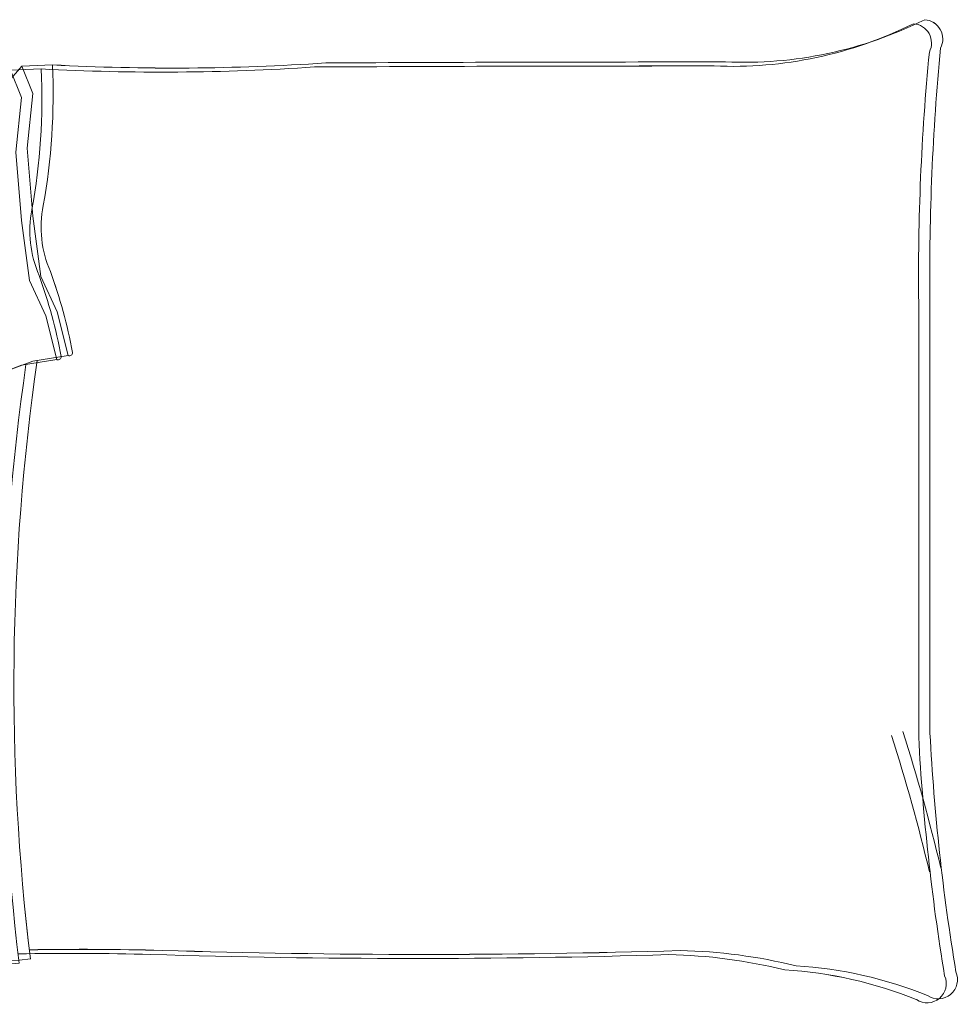
# Model space of a CAD drawing. Units: inches. Extents: x 1962 to 2771, y 1245 to 2660.
# Tile 27 of 114: x 2116 to 2158, y 1849 to 1893. Entities that reach past the tile are written whole.
import ezdxf

# ---------------------------------------------------------------- set-up
doc = ezdxf.new("R2010")
doc.units = ezdxf.units.IN
doc.layers.add('A-FURN', color=8, linetype='Continuous', lineweight=13)

# ---------------------------------------------------------------- blocks, each defined once
blk = doc.blocks.new('BED-PLAN')
for p, q in [((22.563, 42.207), (19.979, 39.261)), ((22.563, 42.206), (19.979, 39.261)), ((23.95, 42.27), (22.563, 42.207, 3.077)), ((23.95, 42.27), (22.563, 42.206, 3.077)), ((23.055, 40.985), (22.563, 42.207)), ((23.055, 40.985), (22.563, 42.206)), ((22.055, 42.025), (19.471, 39.08)), ((22.055, 42.025), (19.471, 39.08)), ((23.442, 42.088), (22.055, 42.025, 3.077)), ((23.442, 42.088), (22.055, 42.025, 3.077)), ((22.547, 40.803), (22.055, 42.025)), ((22.547, 40.803), (22.055, 42.025)), ((0.508, 40.933), (21.66, 40.933)), ((0.508, 40.933), (21.66, 40.933)), ((1.727, 2.945), (1.727, 40.933)), ((1.727, 2.945), (1.727, 40.933)), ((22.809, 38.523), (23.055, 40.985)), ((22.809, 38.522), (23.055, 40.985)), ((0, 40.752), (21.152, 40.752)), ((0, 40.751), (21.152, 40.751)), ((0, 2.764), (0, 40.751)), ((1.219, 2.764), (1.219, 40.752)), ((1.219, 2.763), (1.219, 40.751)), ((13.682, 40.482), (11.187, 39.866)), ((13.682, 40.482), (11.187, 39.866)), ((13.361, 36.403), (13.682, 40.482)), ((13.361, 36.403), (13.682, 40.482)), ((22.301, 38.341), (22.547, 40.803)), ((22.301, 38.341), (22.547, 40.803)), ((2.541, 40.016), (2.464, 35.722)), ((2.541, 40.016), (2.464, 35.722)), ((2.541, 40.016), (5.093, 39.715)), ((2.541, 40.016), (5.093, 39.715)), ((4.585, 39.534), (6.628, 40.007)), ((4.585, 39.533), (6.628, 40.007)), ((5.093, 39.715), (7.136, 40.188)), ((5.093, 39.715), (7.136, 40.188)), ((6.628, 40.007), (7.46, 39.598)), ((6.628, 40.007), (7.46, 39.598)), ((9.911, 40.016), (7.072, 39.378)), ((9.911, 40.016), (7.072, 39.378)), ((7.136, 40.188), (7.968, 39.78)), ((7.136, 40.188), (7.968, 39.78)), ((11.187, 39.866), (9.911, 40.016)), ((11.187, 39.866), (9.911, 40.016)), ((13.173, 40.301), (10.679, 39.684)), ((13.173, 40.301), (10.679, 39.684)), ((12.853, 36.222), (13.173, 40.301)), ((12.853, 36.221), (13.173, 40.301)), ((2.033, 39.835), (1.955, 35.54)), ((2.033, 39.834), (1.956, 35.54)), ((2.033, 39.835), (4.585, 39.534)), ((2.033, 39.834), (4.585, 39.533)), ((9.402, 39.835), (6.563, 39.197)), ((9.402, 39.835), (6.563, 39.197)), ((10.679, 39.684), (9.402, 39.835)), ((10.679, 39.684), (9.402, 39.835)), ((6.563, 39.197), (4.434, 38.258)), ((6.563, 39.197), (4.434, 38.258)), ((7.072, 39.378), (4.942, 38.439)), ((7.072, 39.378), (4.942, 38.439)), ((19.471, 39.08), (17.749, 36.741)), ((19.471, 39.08), (17.749, 36.741)), ((19.979, 39.261), (18.257, 36.922)), ((19.979, 39.261), (18.257, 36.922)), ((22.547, 35.263), (22.301, 38.341)), ((22.547, 35.263), (22.301, 38.341)), ((23.055, 35.445), (22.809, 38.523)), ((23.055, 35.445), (22.809, 38.522)), ((18.257, 36.922), (16.658, 32.49)), ((18.257, 36.922), (16.658, 32.49)), ((2.464, 35.722), (2.529, 36.519)), ((2.464, 35.722), (2.529, 36.519)), ((2.529, 36.519), (2.948, 33.5)), ((2.529, 36.519), (2.948, 33.5)), ((13.804, 34.845), (13.361, 36.403)), ((13.804, 34.845), (13.361, 36.403)), ((17.749, 36.741), (16.149, 32.309)), ((17.749, 36.741), (16.149, 32.309)), ((1.955, 35.54), (2.021, 36.338)), ((1.956, 35.54), (2.021, 36.337)), ((2.021, 36.338), (2.44, 33.319)), ((2.021, 36.337), (2.44, 33.318)), ((13.296, 34.663), (12.853, 36.222)), ((13.296, 34.663), (12.853, 36.221)), ((22.916, 32.555), (22.547, 35.263)), ((22.916, 32.555), (22.547, 35.263)), ((23.424, 32.737), (23.055, 35.445)), ((23.424, 32.736), (23.055, 35.445)), ((12.953, 29.091), (13.296, 34.663)), ((12.953, 29.091), (13.296, 34.663)), ((13.461, 29.273), (13.804, 34.845)), ((13.461, 29.273), (13.804, 34.845)), ((2.44, 33.319), (3.515, 29.011)), ((2.44, 33.318), (3.515, 29.011)), ((2.948, 33.5), (4.023, 29.192)), ((2.948, 33.5), (4.023, 29.192)), ((16.658, 32.49), (14.326, 25.863)), ((16.658, 32.49), (14.326, 25.862)), ((23.654, 30.955), (22.916, 32.555)), ((23.654, 30.955), (22.916, 32.555)), ((24.162, 31.136), (23.424, 32.737)), ((24.162, 31.136), (23.424, 32.736)), ((16.149, 32.309), (13.818, 25.681)), ((16.149, 32.309), (13.818, 25.681)), ((62.991, 11.975), (62.991, 31.54)), ((62.991, 11.975), (62.991, 31.54)), ((63.499, 12.157), (63.499, 31.722)), ((63.499, 12.156), (63.499, 31.722)), ((2.92, 31.161), (2.447, 29.52)), ((2.92, 31.161), (2.447, 29.519)), ((3.428, 31.343), (2.955, 29.701)), ((3.428, 31.342), (2.955, 29.701)), ((24.655, 29.167), (24.162, 31.136)), ((24.655, 29.166), (24.162, 31.136)), ((24.146, 28.985), (23.654, 30.955)), ((24.146, 28.985), (23.654, 30.955)), ((2.447, 29.52), (2.017, 27.19)), ((2.447, 29.519), (2.017, 27.19)), ((2.955, 29.701), (2.525, 27.372)), ((2.955, 29.701), (2.525, 27.372)), ((12.423, 25.886), (12.953, 29.091)), ((12.423, 25.886), (12.953, 29.091)), ((12.931, 26.068), (13.461, 29.273)), ((12.931, 26.068), (13.461, 29.273)), ((19.487, 27.566), (23.055, 28.92)), ((19.487, 27.566), (23.055, 28.92)), ((22.547, 28.739), (24.146, 28.985)), ((22.547, 28.739), (24.146, 28.985)), ((23.055, 28.92), (24.655, 29.167)), ((23.055, 28.92), (24.655, 29.166)), ((18.979, 27.385), (22.547, 28.739)), ((18.979, 27.384), (22.547, 28.739)), ((14.326, 24.236), (19.487, 27.566)), ((14.326, 24.235), (19.487, 27.566)), ((2.017, 27.19), (2.033, 26.935)), ((2.017, 27.19), (2.033, 26.935)), ((2.525, 27.372), (2.541, 27.117)), ((2.525, 27.372), (2.541, 27.116)), ((2.541, 27.117), (2.876, 23.597)), ((2.541, 27.116), (2.876, 23.597)), ((13.818, 24.054), (18.979, 27.385)), ((13.818, 24.054), (18.979, 27.384)), ((2.033, 26.935), (2.368, 23.415)), ((2.033, 26.935), (2.368, 23.415)), ((13.306, 24.444), (12.285, 26.885)), ((13.306, 24.444), (12.285, 26.885)), ((13.814, 24.626), (12.793, 27.067)), ((13.814, 24.626), (12.793, 27.066)), ((13.428, 22.495), (13.306, 24.444)), ((13.428, 22.495), (13.306, 24.444)), ((13.936, 22.676), (13.814, 24.626)), ((13.936, 22.676), (13.814, 24.626)), ((2.876, 23.597), (2.489, 22.421)), ((2.876, 23.597), (2.489, 22.421)), ((2.368, 23.415), (1.981, 22.24)), ((2.368, 23.415), (1.981, 22.24)), ((11.809, 22.543), (13.936, 22.676)), ((11.809, 22.543), (13.936, 22.676)), ((1.981, 22.24), (6.254, 22.046)), ((1.981, 22.24), (6.254, 22.046)), ((2.489, 22.421), (6.762, 22.228)), ((2.489, 22.421), (6.762, 22.228)), ((6.762, 22.228), (9.314, 21.927)), ((6.762, 22.228), (9.314, 21.927)), ((9.838, 21.81), (11.301, 22.362)), ((9.838, 21.81), (11.301, 22.362)), ((10.346, 21.991), (11.809, 22.543)), ((10.346, 21.991), (11.809, 22.543)), ((11.301, 22.362), (13.428, 22.495)), ((11.301, 22.362), (13.428, 22.495)), ((6.247, 21.296), (8.776, 21.755)), ((6.247, 21.296), (8.776, 21.755)), ((6.254, 22.046), (8.806, 21.745)), ((6.254, 22.046), (8.806, 21.745)), ((8.776, 21.755), (9.81, 21.755)), ((8.776, 21.755), (9.81, 21.755)), ((8.806, 21.745), (9.838, 21.81)), ((8.806, 21.745), (9.838, 21.81)), ((9.314, 21.927), (10.346, 21.991)), ((9.314, 21.927), (10.346, 21.991)), ((9.81, 21.755), (11.304, 21.296)), ((9.81, 21.755), (11.304, 21.296)), ((5.739, 21.114), (8.268, 21.574)), ((5.739, 21.114), (8.268, 21.574)), ((8.268, 21.574), (9.302, 21.574)), ((8.268, 21.574), (9.302, 21.574)), ((9.302, 21.574), (10.796, 21.114)), ((9.302, 21.574), (10.796, 21.114)), ((1.487, 20.655), (5.739, 21.114)), ((1.487, 20.654), (5.739, 21.114)), ((1.995, 20.836), (6.247, 21.296)), ((1.995, 20.836), (6.247, 21.296)), ((10.796, 21.114), (12.927, 21.114)), ((10.796, 21.114), (12.927, 21.114)), ((11.304, 21.296), (13.436, 21.296)), ((11.304, 21.296), (13.436, 21.296)), ((12.927, 21.114), (12.927, 19.161)), ((12.927, 21.114), (12.927, 19.161)), ((13.436, 21.296), (13.436, 19.342)), ((13.436, 21.296), (13.436, 19.342)), ((1.946, 19.506), (1.487, 20.655)), ((1.946, 19.505), (1.487, 20.654)), ((2.455, 19.687), (1.995, 20.836)), ((2.455, 19.687), (1.995, 20.836)), ((2.34, 16.153), (2.455, 19.687)), ((2.34, 16.153), (2.455, 19.687)), ((13.361, 15.591), (13.682, 19.67)), ((13.361, 15.591), (13.682, 19.67)), ((1.831, 15.972), (1.946, 19.506)), ((1.831, 15.972), (1.946, 19.505)), ((12.927, 19.161), (12.06, 16.661)), ((12.927, 19.161), (12.06, 16.661)), ((13.436, 19.342), (12.568, 16.843)), ((13.436, 19.342), (12.568, 16.843)), ((12.853, 15.409), (13.173, 19.489)), ((12.853, 15.409), (13.173, 19.488)), ((2.34, 15.898), (2.34, 16.153)), ((2.34, 15.897), (2.34, 16.153)), ((1.831, 15.716), (1.831, 15.972)), ((1.831, 15.716), (1.831, 15.972)), ((2.406, 13.418), (1.831, 15.716)), ((2.406, 13.418), (1.831, 15.716)), ((2.914, 13.6), (2.34, 15.898)), ((2.914, 13.599), (2.34, 15.897)), ((13.804, 14.033), (13.361, 15.591)), ((13.804, 14.032), (13.361, 15.591)), ((13.296, 13.851), (12.853, 15.409)), ((13.296, 13.851), (12.853, 15.409)), ((2.636, 9.626), (3.44, 13.993)), ((2.636, 9.626), (3.44, 13.992)), ((3.144, 9.808), (3.949, 14.174)), ((3.144, 9.807), (3.949, 14.174)), ((12.953, 8.279), (13.296, 13.851)), ((12.953, 8.279), (13.296, 13.851)), ((13.461, 8.461), (13.804, 14.033)), ((13.461, 8.46), (13.804, 14.032)), ((2.981, 11.809), (2.406, 13.418)), ((2.981, 11.809), (2.406, 13.418)), ((3.489, 11.991), (2.914, 13.6)), ((3.489, 11.991), (2.914, 13.599)), ((2.914, 6.768), (3.144, 9.808)), ((2.914, 6.768), (3.144, 9.807)), ((2.406, 6.587), (2.636, 9.626)), ((2.406, 6.587), (2.636, 9.626)), ((12.931, 5.256), (13.461, 8.461)), ((12.931, 5.255), (13.461, 8.46)), ((13.461, 8.461), (13.718, 7.56)), ((13.461, 8.46), (13.718, 7.56)), ((12.423, 5.074), (12.953, 8.279)), ((12.423, 5.074), (12.953, 8.279)), ((12.953, 8.279), (13.21, 7.378)), ((12.953, 8.279), (13.21, 7.378)), ((13.718, 7.56), (14.292, 3.509)), ((13.718, 7.56), (14.292, 3.508)), ((13.21, 7.378), (13.784, 3.327)), ((13.21, 7.378), (13.784, 3.327)), ((2.9, 6.685), (2.914, 6.768)), ((2.9, 6.684), (2.914, 6.768)), ((3.162, 3.282), (2.9, 6.685)), ((3.162, 3.282), (2.9, 6.684)), ((2.392, 6.503), (2.406, 6.587)), ((2.392, 6.503), (2.406, 6.587)), ((2.653, 3.1), (2.392, 6.503)), ((2.653, 3.1), (2.392, 6.503)), ((7.626, 4.198), (5.443, 5.002)), ((7.626, 4.198), (5.443, 5.002)), ((7.118, 4.016), (4.935, 4.821)), ((7.118, 4.016), (4.935, 4.821)), ((9.991, 3.557), (7.118, 4.016)), ((9.992, 3.557), (7.118, 4.016)), ((10.5, 3.738), (7.626, 4.198)), ((10.5, 3.738), (7.626, 4.198)), ((2.636, 3.097), (5.164, 3.557)), ((2.636, 3.097), (5.164, 3.557)), ((3.144, 3.279), (5.673, 3.738)), ((3.144, 3.279), (5.673, 3.738)), ((5.164, 3.557), (7.233, 3.212)), ((5.164, 3.557), (7.233, 3.212)), ((5.673, 3.738), (7.741, 3.394)), ((5.673, 3.738), (7.741, 3.393)), ((7.233, 3.212), (8.038, 3.672)), ((7.233, 3.212), (8.038, 3.672)), ((7.741, 3.394), (8.546, 3.853)), ((7.741, 3.393), (8.546, 3.853)), ((11.256, 3.787), (9.991, 3.557)), ((11.256, 3.786), (9.992, 3.557)), ((11.764, 3.968), (10.5, 3.738)), ((11.764, 3.968), (10.5, 3.738)), ((13.784, 3.327), (11.256, 3.787)), ((13.784, 3.327), (11.256, 3.786)), ((14.292, 3.509), (11.764, 3.968)), ((14.292, 3.508), (11.764, 3.968)), ((14.396, 2.764), (0, 2.764)), ((14.396, 2.763), (0, 2.763)), ((14.904, 2.945), (0.508, 2.945)), ((14.904, 2.945), (0.508, 2.945))]:
    blk.add_line(p, q)
for centre, radius, start, end in [((54.582, 60.538), 18.334, 267.4714, 296.4681), ((54.582, 60.538), 18.334, 267.4714, 296.4681), ((55.09, 60.719), 18.334, 267.4714, 296.4681), ((55.09, 60.719), 18.334, 267.4714, 296.4681), ((62.693, 43.251), 0.876, 332.6588, 86.02), ((62.693, 43.251), 0.876, 332.6588, 86.02), ((63.201, 43.433), 0.876, 332.6588, 86.02), ((63.201, 43.432), 0.876, 332.6588, 86.02), ((168.736, 32.712), 105.752, 174.4998, 180.63509), ((168.736, 32.712), 105.752, 174.4998, 180.63509), ((169.244, 32.894), 105.752, 174.4998, 180.63509), ((169.244, 32.894), 105.752, 174.4998, 180.63509), ((28.866, 144.882), 102.937, 266.97912, 273.83645), ((28.866, 144.882), 102.937, 266.97912, 273.83645), ((-4.783, 40.982), 28.761, 349.8763, 2.5657), ((-4.783, 40.982), 28.761, 349.8763, 2.5657), ((29.375, 145.064), 102.937, 266.97912, 273.83645), ((29.375, 145.063), 102.937, 266.97912, 273.83645), ((53.91, -3583.936), 3626.158, 90.002168, 90.286887), ((53.91, -3583.937), 3626.158, 90.002168, 90.286887), ((54.419, -3583.755), 3626.158, 90.002168, 90.286887), ((54.419, -3583.755), 3626.158, 90.002168, 90.286887), ((-5.291, 40.801), 28.761, 349.8763, 2.5657), ((-5.291, 40.801), 28.761, 349.8763, 2.5657), ((27.874, 34.772), 4.948, 168.6608, 203.7384), ((27.874, 34.772), 4.948, 168.6608, 203.7384), ((28.382, 34.954), 4.948, 168.6608, 203.7384), ((28.382, 34.954), 4.948, 168.6608, 203.7384), ((1.686, 24.947), 23.571, 10.6617, 19.8806), ((1.686, 24.946), 23.571, 10.6617, 19.8806), ((1.178, 24.765), 23.571, 10.6617, 19.8806), ((1.178, 24.765), 23.571, 10.6617, 19.8806), ((24.704, 29.305), 0.147, 250.2464, 1.1377), ((24.704, 29.304), 0.147, 250.2464, 1.1377), ((124.762, 14.297), 102.556, 171.78449, 186.90062), ((124.762, 14.296), 102.556, 171.78449, 186.90062), ((24.196, 29.123), 0.147, 250.2464, 1.1377), ((24.196, 29.123), 0.147, 250.2464, 1.1377), ((124.254, 14.115), 102.556, 171.78449, 186.90062), ((124.254, 14.115), 102.556, 171.78449, 186.90062), ((144.711, 16.979), 131.131, 176.08655, 186.78213), ((144.711, 16.979), 131.131, 176.08655, 186.78213), ((145.219, 17.161), 131.131, 176.08655, 186.78213), ((145.219, 17.161), 131.131, 176.08655, 186.78213), ((-18.848, -13.688), 84.623, 13.38322, 17.70533), ((-18.848, -13.688), 84.623, 13.38322, 17.70533), ((-18.34, -13.506), 84.623, 13.38322, 17.70533), ((-18.34, -13.507), 84.623, 13.38322, 17.70533), ((160.151, 17.215), 96.784, 182.99578, 189.40907), ((160.151, 17.215), 96.784, 182.99578, 189.40907), ((159.643, 17.033), 96.784, 182.99578, 189.40907), ((159.643, 17.033), 96.784, 182.99578, 189.40907), ((24.78, -132.989), 135.218, 88.4762, 91.00819), ((24.78, -132.989), 135.218, 88.4762, 91.00819), ((25.288, -132.807), 135.218, 88.4762, 91.00819), ((25.288, -132.808), 135.218, 88.4762, 91.00819), ((40.74, 385.562), 383.382, 268.22771, 271.71854), ((40.74, 385.561), 383.382, 268.22771, 271.71854), ((51.79, -21.199), 23.556, 76.0648, 88.9113), ((51.79, -21.199), 23.556, 76.0648, 88.9113), ((15.974, 67.695), 66.218, 268.72178, 275.60397), ((15.974, 67.695), 66.218, 268.72178, 275.60397), ((16.482, 67.877), 66.218, 268.72178, 275.60397), ((16.483, 67.877), 66.218, 268.72178, 275.60397), ((40.232, 385.38), 383.382, 268.22771, 271.71854), ((40.232, 385.38), 383.382, 268.22771, 271.71854), ((51.282, -21.381), 23.556, 76.0648, 88.9113), ((51.282, -21.381), 23.556, 76.0648, 88.9113), ((55.861, -17.215), 18.729, 67.9751, 86.652), ((55.861, -17.216), 18.729, 67.9751, 86.652), ((56.369, -17.034), 18.729, 67.9751, 86.652), ((56.369, -17.034), 18.729, 67.9751, 86.652), ((63.875, 1.047), 0.866, 236.1736, 23.4781), ((63.875, 1.047), 0.866, 236.1736, 23.4781), ((63.367, 0.866), 0.866, 236.1736, 23.4781), ((63.367, 0.866), 0.866, 236.1736, 23.4781)]:
    blk.add_arc(centre, radius, start, end)

msp = doc.modelspace()

# ---------------------------------------------------------------- block references
at = {"layer": 'A-FURN'}
msp.add_blockref('BED-PLAN', (2093.6551, 1848.7344), dxfattribs=at)

doc.saveas('drawing.dxf')
